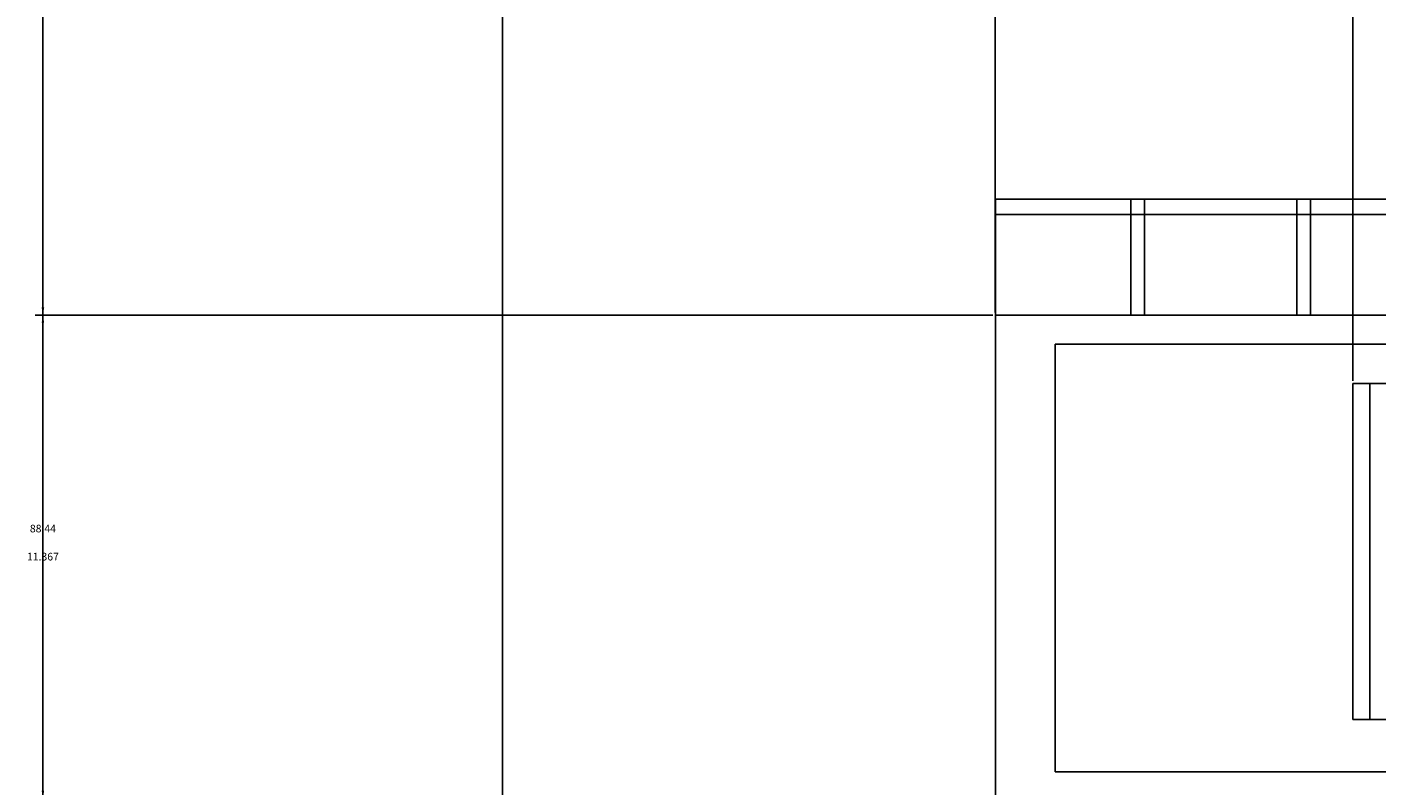
# Model space of a CAD drawing. Units: inches. Extents: x -117 to 121, y -77 to 40.
# Tile 9 of 45: x -117 to -85, y -23 to -5. Entities that reach past the tile are written whole.
import ezdxf

# ---------------------------------------------------------------- set-up
doc = ezdxf.new("R2010")
doc.units = ezdxf.units.IN
doc.header["$MEASUREMENT"] = 0
doc.layers.add('A-ANNO-DIMS', color=2, linetype='Continuous', lineweight=18)
doc.layers.add('A-ELEV', color=7, linetype='Continuous', lineweight=25)
doc.styles.get("Standard").update_dxf_attribs({"font": 'arial.ttf'})
doc.dimstyles.get("Standard").update_dxf_attribs({"dimtxt": 0.18, "dimasz": 0.18, "dimexe": 0.18, "dimexo": 0.0625, "dimgap": 0.09, "dimtad": 0, "dimtih": 1, "dimtoh": 1, "dimdec": 4, "dimzin": 0, "dimdsep": 46, "dimtxsty": 'Standard', "dimcen": 0.09, "dimadec": 0, "dimazin": 0, "dimtfac": 1, "dimtdec": 4, "dimtofl": 0, "dimtmove": 0, "dimatfit": 3, "dimfxl": 1, "dimtolj": 1, "dimtzin": 0, "dimarcsym": 0})

# ---------------------------------------------------------------- blocks, each defined once
blk = doc.blocks.new('*D13')
at = {"layer": 'A-ANNO-DIMS', "color": 0, "lineweight": -2, "transparency": 16777216}
for p, q in [((-2.663, 27.063), (-117.024, 27.063)), ((-116.844, 26.883), (-116.844, -16.974)), ((-116.844, -61.196), (-116.844, -17.338)), ((-106.096, -61.376), (-117.024, -61.376))]:
    blk.add_line(p, q, dxfattribs=at)
at = {"layer": 'A-ANNO-DIMS', "color": 0, "transparency": 16777216}
for points in [[(-116.874, 26.883), (-116.814, 26.883), (-116.844, 27.063)], [(-116.874, -61.196), (-116.814, -61.196), (-116.844, -61.376)]]:
    blk.add_solid(points, dxfattribs=at)
at = {"layer": 'Defpoints', "color": 0, "transparency": 16777216}
for p in [(-2.6, 27.063), (-116.844, -61.376), (-106.034, -61.376)]:
    blk.add_point(p, dxfattribs=at)
at = {"layer": 'A-ANNO-DIMS', "color": 0, "transparency": 16777216, "insert": (-116.844, -17.156), "char_height": 0.18, "attachment_point": 5}
blk.add_mtext('\\A1;88.44', dxfattribs=at)
blk = doc.blocks.new('*D19')
at = {"layer": 'A-ANNO-DIMS', "color": 0, "lineweight": -2, "transparency": 16777216}
for p, q in [((-94.498, -12.133), (-117.024, -12.133)), ((-116.844, -12.313), (-116.844, -17.635)), ((-116.844, -23.321), (-116.844, -17.999)), ((-94.498, -23.501), (-117.024, -23.501))]:
    blk.add_line(p, q, dxfattribs=at)
at = {"layer": 'A-ANNO-DIMS', "color": 0, "transparency": 16777216}
for points in [[(-116.874, -12.313), (-116.814, -12.313), (-116.844, -12.133)], [(-116.874, -23.321), (-116.814, -23.321), (-116.844, -23.501)]]:
    blk.add_solid(points, dxfattribs=at)
at = {"layer": 'Defpoints', "color": 0, "transparency": 16777216}
for p in [(-94.436, -12.133), (-116.844, -23.501), (-94.436, -23.501)]:
    blk.add_point(p, dxfattribs=at)
at = {"layer": 'A-ANNO-DIMS', "color": 0, "transparency": 16777216, "insert": (-116.844, -17.817), "char_height": 0.18, "attachment_point": 5}
blk.add_mtext('\\A1;11.367', dxfattribs=at)
blk = doc.blocks.new('*D20')
at = {"layer": 'A-ANNO-DIMS', "color": 0, "lineweight": -2, "transparency": 16777216}
for p, q in [((-75.866, 11.871), (-117.024, 11.871)), ((-116.844, 11.691), (-116.844, 0.051)), ((-116.844, -11.953), (-116.844, -0.313)), ((-94.498, -12.133), (-117.024, -12.133))]:
    blk.add_line(p, q, dxfattribs=at)
at = {"layer": 'A-ANNO-DIMS', "color": 0, "transparency": 16777216}
for points in [[(-116.874, 11.691), (-116.814, 11.691), (-116.844, 11.871)], [(-116.874, -11.953), (-116.814, -11.953), (-116.844, -12.133)]]:
    blk.add_solid(points, dxfattribs=at)
at = {"layer": 'Defpoints', "color": 0, "transparency": 16777216}
for p in [(-75.804, 11.871), (-116.844, -12.133), (-94.436, -12.133)]:
    blk.add_point(p, dxfattribs=at)
at = {"layer": 'A-ANNO-DIMS', "color": 0, "transparency": 16777216, "insert": (-116.844, -0.131), "char_height": 0.18, "attachment_point": 5}
blk.add_mtext('\\A1;24.004', dxfattribs=at)
blk = doc.blocks.new('*D21')
at = {"layer": 'A-ANNO-DIMS', "color": 0, "lineweight": -2, "transparency": 16777216}
for p, q in [((-106.034, -61.313), (-106.034, 38.61)), ((-75.804, 8.087), (-75.804, 38.61)), ((-105.854, 38.43), (-91.382, 38.43)), ((-75.984, 38.43), (-90.455, 38.43))]:
    blk.add_line(p, q, dxfattribs=at)
at = {"layer": 'A-ANNO-DIMS', "color": 0, "transparency": 16777216}
for points in [[(-105.854, 38.46), (-105.854, 38.4), (-106.034, 38.43)], [(-75.984, 38.46), (-75.984, 38.4), (-75.804, 38.43)]]:
    blk.add_solid(points, dxfattribs=at)
at = {"layer": 'Defpoints', "color": 0, "transparency": 16777216}
for p in [(-75.804, 38.43), (-75.804, 8.025), (-106.034, -61.376)]:
    blk.add_point(p, dxfattribs=at)
at = {"layer": 'A-ANNO-DIMS', "color": 0, "transparency": 16777216, "insert": (-90.919, 38.43), "char_height": 0.18, "attachment_point": 5}
blk.add_mtext('\\A1;30.230', dxfattribs=at)
blk = doc.blocks.new('*D39')
at = {"layer": 'A-ANNO-DIMS', "color": 0, "lineweight": -2, "transparency": 16777216}
for p, q in [((-94.436, -12.071), (-94.436, 38.61)), ((-86.023, -13.677), (-86.023, 38.61)), ((-94.256, 38.43), (-90.623, 38.43)), ((-86.203, 38.43), (-89.835, 38.43))]:
    blk.add_line(p, q, dxfattribs=at)
at = {"layer": 'A-ANNO-DIMS', "color": 0, "transparency": 16777216}
for points in [[(-94.256, 38.46), (-94.256, 38.4), (-94.436, 38.43)], [(-86.203, 38.46), (-86.203, 38.4), (-86.023, 38.43)]]:
    blk.add_solid(points, dxfattribs=at)
at = {"layer": 'Defpoints', "color": 0, "transparency": 16777216}
for p in [(-86.023, 38.43), (-94.436, -12.133), (-86.023, -13.74)]:
    blk.add_point(p, dxfattribs=at)
at = {"layer": 'A-ANNO-DIMS', "color": 0, "transparency": 16777216, "insert": (-90.229, 38.43), "char_height": 0.18, "attachment_point": 5}
blk.add_mtext('\\A1;8.413', dxfattribs=at)
blk = doc.blocks.new('*D40')
at = {"layer": 'A-ANNO-DIMS', "color": 0, "lineweight": -2, "transparency": 16777216}
for p, q in [((-86.023, -13.677), (-86.023, 38.61)), ((-63.159, -13.677), (-63.159, 38.61)), ((-85.843, 38.43), (-75.056, 38.43)), ((-63.339, 38.43), (-74.126, 38.43))]:
    blk.add_line(p, q, dxfattribs=at)
at = {"layer": 'A-ANNO-DIMS', "color": 0, "transparency": 16777216}
for points in [[(-85.843, 38.46), (-85.843, 38.4), (-86.023, 38.43)], [(-63.339, 38.46), (-63.339, 38.4), (-63.159, 38.43)]]:
    blk.add_solid(points, dxfattribs=at)
at = {"layer": 'Defpoints', "color": 0, "transparency": 16777216}
for p in [(-63.159, 38.43), (-86.023, -13.74), (-63.159, -13.74)]:
    blk.add_point(p, dxfattribs=at)
at = {"layer": 'A-ANNO-DIMS', "color": 0, "transparency": 16777216, "insert": (-74.591, 38.43), "char_height": 0.18, "attachment_point": 5}
blk.add_mtext('\\A1;22.864', dxfattribs=at)

msp = doc.modelspace()

# ---------------------------------------------------------------- linework, layer by layer
at = {"layer": 'A-ELEV'}
for p, q in [((-94.4355, -12.1334), (-94.4355, -9.4047)), ((-94.4355, -9.4047), (-75.8037, -9.4047)), ((-91.2459, -12.1334), (-91.2459, -9.4047)), ((-90.927, -12.1334), (-90.927, -9.4047)), ((-87.3386, -12.1334), (-87.3386, -9.4047)), ((-87.0197, -12.1334), (-87.0197, -9.4047)), ((-94.4355, -9.7631), (-75.8037, -9.7631)), ((-64.513, -12.1334), (-94.4355, -12.1334)), ((-94.4355, -23.5007), (-94.4355, -12.1334)), ((-64.513, -12.8131), (-93.028, -12.8131)), ((-93.028, -22.8827), (-93.028, -12.8131)), ((-64.513, -13.74), (-86.0225, -13.74)), ((-86.0225, -21.6476), (-86.0225, -13.74)), ((-85.6266, -21.6476), (-85.6266, -13.74)), ((-64.513, -21.6476), (-86.0225, -21.6476)), ((-46.5108, -22.8827), (-93.028, -22.8827))]:
    msp.add_line(p, q, dxfattribs=at)

# ---------------------------------------------------------------- dimensions: what is measured, and where the dimension line sits
at = {"layer": 'A-ANNO-DIMS'}
for base, p1, p2, picture, middle in [((-75.8037, 38.4297), (-106.0338, -61.3756), (-75.8037, 8.0246), '*D21', (-90.9187, 38.4297)), ((-86.0225, 38.4297), (-94.4355, -12.1334), (-86.0225, -13.74), '*D39', (-90.229, 38.4297)), ((-63.1589, 38.4297), (-86.0225, -13.74), (-63.1589, -13.74), '*D40', (-74.5907, 38.4297))]:
    dim = msp.add_linear_dim(base=base, p1=p1, p2=p2, dimstyle='Standard', override={"dimdec": 3, "dimlfac": 1, "dimrnd": 0, "dimzin": 0, "dimdsep": 46, "dimlunit": 2}, dxfattribs=at)
    dim.commit()
    dim.dimension.update_dxf_attribs({"geometry": picture, "text_midpoint": middle})
for base, p1, p2, override, picture, middle in [((-116.8438, -61.3756), (-2.6001, 27.0634), (-106.0338, -61.3756), {"dimdec": 2, "dimlfac": 1, "dimrnd": 0, "dimzin": 0, "dimdsep": 46, "dimlunit": 2}, '*D13', (-116.8438, -17.1561)), ((-116.84377, -12.13336), (-75.80372, 11.87111), (-94.43553, -12.13336), {"dimdec": 3, "dimlfac": 1, "dimrnd": 0, "dimzin": 0, "dimdsep": 46, "dimlunit": 2}, '*D20', (-116.84377, -0.13113)), ((-116.8438, -23.5007), (-94.4355, -12.1334), (-94.4355, -23.5007), {"dimdec": 3, "dimlfac": 1, "dimrnd": 0, "dimzin": 0, "dimdsep": 46, "dimlunit": 2}, '*D19', (-116.8438, -17.817))]:
    dim = msp.add_linear_dim(base=base, p1=p1, p2=p2, angle=90, dimstyle='Standard', override=override, dxfattribs=at)
    dim.commit()
    dim.dimension.update_dxf_attribs({"geometry": picture, "text_midpoint": middle})

doc.saveas('drawing.dxf')
